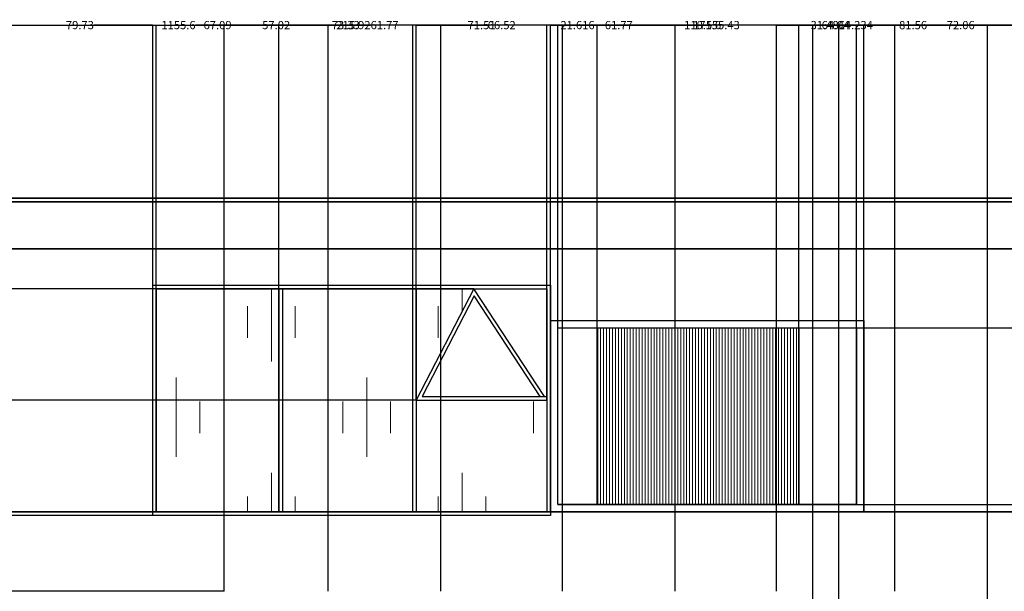
# Model space of a CAD drawing. Units: inches. Extents: x -1308 to 780, y 304 to 1023.
# Tile 6 of 7: x -138 to 402, y 709 to 1023. Entities that reach past the tile are written whole.
import ezdxf

# ---------------------------------------------------------------- set-up
doc = ezdxf.new("R2010")
doc.units = ezdxf.units.IN
doc.header["$MEASUREMENT"] = 0
for name, color, linetype, lineweight in [('A-ANNO-DIMS', 2, 'Continuous', 18), ('A-ELEV', 7, 'Continuous', 35), ('A-ELEV-PATT', 8, 'Continuous', 13), ('A-GLAZ', 4, 'Continuous', 25)]:
    doc.layers.add(name, color=color, linetype=linetype, lineweight=lineweight)
doc.styles.get("Standard").update_dxf_attribs({"font": 'arial.ttf'})
doc.dimstyles.get("Standard").update_dxf_attribs({"dimtxt": 4.5, "dimasz": 0.18, "dimexe": 0.18, "dimexo": 0.0625, "dimgap": 0.09, "dimtad": 0, "dimtih": 1, "dimtoh": 1, "dimdec": 4, "dimzin": 0, "dimdsep": 46, "dimlunit": 4, "dimtxsty": 'Standard', "dimcen": 0.09, "dimadec": 0, "dimazin": 0, "dimtfac": 1, "dimtdec": 4, "dimtofl": 0, "dimtmove": 0, "dimatfit": 3, "dimfxl": 1, "dimtolj": 1, "dimtzin": 0, "dimarcsym": 0})

# ---------------------------------------------------------------- blocks, each defined once
blk = doc.blocks.new('*D18')
at = {"layer": 'A-ANNO-DIMS', "color": 0, "lineweight": -2, "transparency": 16777216}
for p, q in [((-628.68, 924.9), (-628.68, 1019.77)), ((-628.5, 1019.59), (-60.08, 1019.59)), ((526.78, 1019.59), (-41.64, 1019.59)), ((526.96, 924.9), (526.96, 1019.77))]:
    blk.add_line(p, q, dxfattribs=at)
at = {"layer": 'A-ANNO-DIMS', "color": 0, "transparency": 16777216}
for points in [[(-628.5, 1019.62), (-628.5, 1019.56), (-628.68, 1019.59)], [(526.78, 1019.62), (526.78, 1019.56), (526.96, 1019.59)]]:
    blk.add_solid(points, dxfattribs=at)
at = {"layer": 'Defpoints', "color": 0, "transparency": 16777216}
for p in [(526.96, 1019.59), (-628.68, 924.84), (526.96, 924.84)]:
    blk.add_point(p, dxfattribs=at)
at = {"layer": 'A-ANNO-DIMS', "color": 0, "transparency": 16777216, "insert": (-50.86, 1019.59), "char_height": 4.5, "attachment_point": 5}
blk.add_mtext('\\A1;1155.6', dxfattribs=at)
blk = doc.blocks.new('*D27')
at = {"layer": 'A-ANNO-DIMS', "color": 0, "lineweight": -2, "transparency": 16777216}
for p, q in [((-144.73, 753.1), (-144.73, 1019.77)), ((-144.55, 1019.59), (-112.53, 1019.59)), ((-65.19, 1019.59), (-97.21, 1019.59)), ((-65.01, 751.1), (-65.01, 1019.77))]:
    blk.add_line(p, q, dxfattribs=at)
at = {"layer": 'A-ANNO-DIMS', "color": 0, "transparency": 16777216}
for points in [[(-144.55, 1019.62), (-144.55, 1019.56), (-144.73, 1019.59)], [(-65.19, 1019.62), (-65.19, 1019.56), (-65.01, 1019.59)]]:
    blk.add_solid(points, dxfattribs=at)
at = {"layer": 'Defpoints', "color": 0, "transparency": 16777216}
for p in [(-65.01, 1019.59), (-144.73, 753.04), (-65.01, 751.04)]:
    blk.add_point(p, dxfattribs=at)
at = {"layer": 'A-ANNO-DIMS', "color": 0, "transparency": 16777216, "insert": (-104.87, 1019.59), "char_height": 4.5, "attachment_point": 5}
blk.add_mtext('\\A1;79.73', dxfattribs=at)
blk = doc.blocks.new('*D28')
at = {"layer": 'A-ANNO-DIMS', "color": 0, "lineweight": -2, "transparency": 16777216}
for p, q in [((-63.01, 875.23), (-63.01, 1019.77)), ((-62.83, 1019.59), (35.51, 1019.59)), ((152.73, 1019.59), (54.4, 1019.59)), ((152.91, 877.23), (152.91, 1019.77))]:
    blk.add_line(p, q, dxfattribs=at)
at = {"layer": 'A-ANNO-DIMS', "color": 0, "transparency": 16777216}
for points in [[(-62.83, 1019.62), (-62.83, 1019.56), (-63.01, 1019.59)], [(152.73, 1019.62), (152.73, 1019.56), (152.91, 1019.59)]]:
    blk.add_solid(points, dxfattribs=at)
at = {"layer": 'Defpoints', "color": 0, "transparency": 16777216}
for p in [(152.91, 1019.59), (-63.01, 875.17), (152.91, 877.17)]:
    blk.add_point(p, dxfattribs=at)
at = {"layer": 'A-ANNO-DIMS', "color": 0, "transparency": 16777216, "insert": (44.95, 1019.59), "char_height": 4.5, "attachment_point": 5}
blk.add_mtext('\\A1;215.92', dxfattribs=at)
blk = doc.blocks.new('*D29')
at = {"layer": 'A-ANNO-DIMS', "color": 0, "lineweight": -2, "transparency": 16777216}
for p, q in [((-63.01, 753.1), (-63.01, 1019.77)), ((-62.83, 1019.59), (-37.16, 1019.59)), ((3.9, 1019.59), (-21.76, 1019.59)), ((4.08, 753.1), (4.08, 1019.77))]:
    blk.add_line(p, q, dxfattribs=at)
at = {"layer": 'A-ANNO-DIMS', "color": 0, "transparency": 16777216}
for points in [[(-62.83, 1019.62), (-62.83, 1019.56), (-63.01, 1019.59)], [(3.9, 1019.62), (3.9, 1019.56), (4.08, 1019.59)]]:
    blk.add_solid(points, dxfattribs=at)
at = {"layer": 'Defpoints', "color": 0, "transparency": 16777216}
for p in [(4.08, 1019.59), (-63.01, 753.04), (4.08, 753.04)]:
    blk.add_point(p, dxfattribs=at)
at = {"layer": 'A-ANNO-DIMS', "color": 0, "transparency": 16777216, "insert": (-29.46, 1019.59), "char_height": 4.5, "attachment_point": 5}
blk.add_mtext('\\A1;67.09', dxfattribs=at)
blk = doc.blocks.new('*D30')
at = {"layer": 'A-ANNO-DIMS', "color": 0, "lineweight": -2, "transparency": 16777216}
for p, q in [((4.08, 753.1), (4.08, 1019.77)), ((4.26, 1019.59), (33.08, 1019.59)), ((77.23, 1019.59), (48.41, 1019.59)), ((77.41, 753.1), (77.41, 1019.77))]:
    blk.add_line(p, q, dxfattribs=at)
at = {"layer": 'A-ANNO-DIMS', "color": 0, "transparency": 16777216}
for points in [[(4.26, 1019.62), (4.26, 1019.56), (4.08, 1019.59)], [(77.23, 1019.62), (77.23, 1019.56), (77.41, 1019.59)]]:
    blk.add_solid(points, dxfattribs=at)
at = {"layer": 'Defpoints', "color": 0, "transparency": 16777216}
for p in [(77.41, 1019.59), (4.08, 753.04), (77.41, 753.04)]:
    blk.add_point(p, dxfattribs=at)
at = {"layer": 'A-ANNO-DIMS', "color": 0, "transparency": 16777216, "insert": (40.74, 1019.59), "char_height": 4.5, "attachment_point": 5}
blk.add_mtext('\\A1;73.33', dxfattribs=at)
blk = doc.blocks.new('*D31')
at = {"layer": 'A-ANNO-DIMS', "color": 0, "lineweight": -2, "transparency": 16777216}
for p, q in [((79.41, 814.17), (79.41, 1019.77)), ((79.59, 1019.59), (107.93, 1019.59)), ((150.73, 1019.59), (122.39, 1019.59)), ((150.91, 814.17), (150.91, 1019.77))]:
    blk.add_line(p, q, dxfattribs=at)
at = {"layer": 'A-ANNO-DIMS', "color": 0, "transparency": 16777216}
for points in [[(79.59, 1019.62), (79.59, 1019.56), (79.41, 1019.59)], [(150.73, 1019.62), (150.73, 1019.56), (150.91, 1019.59)]]:
    blk.add_solid(points, dxfattribs=at)
at = {"layer": 'Defpoints', "color": 0, "transparency": 16777216}
for p in [(150.91, 1019.59), (79.41, 814.1), (150.91, 814.1)]:
    blk.add_point(p, dxfattribs=at)
at = {"layer": 'A-ANNO-DIMS', "color": 0, "transparency": 16777216, "insert": (115.16, 1019.59), "char_height": 4.5, "attachment_point": 5}
blk.add_mtext('\\A1;71.51', dxfattribs=at)
blk = doc.blocks.new('*D32')
at = {"layer": 'A-ANNO-DIMS', "color": 0, "lineweight": -2, "transparency": 16777216}
for p, q in [((152.91, 857.81), (152.91, 1019.77)), ((153.09, 1019.59), (231.24, 1019.59)), ((324.33, 1019.59), (246.18, 1019.59)), ((324.51, 857.81), (324.51, 1019.77))]:
    blk.add_line(p, q, dxfattribs=at)
at = {"layer": 'A-ANNO-DIMS', "color": 0, "transparency": 16777216}
for points in [[(153.09, 1019.62), (153.09, 1019.56), (152.91, 1019.59)], [(324.33, 1019.62), (324.33, 1019.56), (324.51, 1019.59)]]:
    blk.add_solid(points, dxfattribs=at)
at = {"layer": 'Defpoints', "color": 0, "transparency": 16777216}
for p in [(324.51, 1019.59), (152.91, 857.74), (324.51, 857.74)]:
    blk.add_point(p, dxfattribs=at)
at = {"layer": 'A-ANNO-DIMS', "color": 0, "transparency": 16777216, "insert": (238.71, 1019.59), "char_height": 4.5, "attachment_point": 5}
blk.add_mtext('\\A1;171.6', dxfattribs=at)
blk = doc.blocks.new('*D33')
at = {"layer": 'A-ANNO-DIMS', "color": 0, "lineweight": -2, "transparency": 16777216}
for p, q in [((156.91, 757.1), (156.91, 1019.77)), ((157.09, 1019.59), (158.26, 1019.59)), ((178.35, 1019.59), (177.19, 1019.59)), ((178.53, 757.1), (178.53, 1019.77))]:
    blk.add_line(p, q, dxfattribs=at)
at = {"layer": 'A-ANNO-DIMS', "color": 0, "transparency": 16777216}
for points in [[(157.09, 1019.62), (157.09, 1019.56), (156.91, 1019.59)], [(178.35, 1019.62), (178.35, 1019.56), (178.53, 1019.59)]]:
    blk.add_solid(points, dxfattribs=at)
at = {"layer": 'Defpoints', "color": 0, "transparency": 16777216}
for p in [(178.53, 1019.59), (156.91, 757.04), (178.53, 757.04)]:
    blk.add_point(p, dxfattribs=at)
at = {"layer": 'A-ANNO-DIMS', "color": 0, "transparency": 16777216, "insert": (167.72, 1019.59), "char_height": 4.5, "attachment_point": 5}
blk.add_mtext('\\A1;21.616', dxfattribs=at)
blk = doc.blocks.new('*D34')
at = {"layer": 'A-ANNO-DIMS', "color": 0, "lineweight": -2, "transparency": 16777216}
for p, q in [((178.53, 757.1), (178.53, 1019.77)), ((178.71, 1019.59), (226.29, 1019.59)), ((288.84, 1019.59), (241.26, 1019.59)), ((289.02, 757.1), (289.02, 1019.77))]:
    blk.add_line(p, q, dxfattribs=at)
at = {"layer": 'A-ANNO-DIMS', "color": 0, "transparency": 16777216}
for points in [[(178.71, 1019.62), (178.71, 1019.56), (178.53, 1019.59)], [(288.84, 1019.62), (288.84, 1019.56), (289.02, 1019.59)]]:
    blk.add_solid(points, dxfattribs=at)
at = {"layer": 'Defpoints', "color": 0, "transparency": 16777216}
for p in [(289.02, 1019.59), (178.53, 757.04), (289.02, 757.04)]:
    blk.add_point(p, dxfattribs=at)
at = {"layer": 'A-ANNO-DIMS', "color": 0, "transparency": 16777216, "insert": (233.78, 1019.59), "char_height": 4.5, "attachment_point": 5}
blk.add_mtext('\\A1;110.5', dxfattribs=at)
blk = doc.blocks.new('*D35')
at = {"layer": 'A-ANNO-DIMS', "color": 0, "lineweight": -2, "transparency": 16777216}
for p, q in [((289.02, 757.1), (289.02, 1019.77)), ((289.2, 1019.59), (295.34, 1019.59)), ((320.33, 1019.59), (314.19, 1019.59)), ((320.51, 757.1), (320.51, 1019.77))]:
    blk.add_line(p, q, dxfattribs=at)
at = {"layer": 'A-ANNO-DIMS', "color": 0, "transparency": 16777216}
for points in [[(289.2, 1019.62), (289.2, 1019.56), (289.02, 1019.59)], [(320.33, 1019.62), (320.33, 1019.56), (320.51, 1019.59)]]:
    blk.add_solid(points, dxfattribs=at)
at = {"layer": 'Defpoints', "color": 0, "transparency": 16777216}
for p in [(320.51, 1019.59), (289.02, 757.04), (320.51, 757.04)]:
    blk.add_point(p, dxfattribs=at)
at = {"layer": 'A-ANNO-DIMS', "color": 0, "transparency": 16777216, "insert": (304.76, 1019.59), "char_height": 4.5, "attachment_point": 5}
blk.add_mtext('\\A1;31.486', dxfattribs=at)
blk = doc.blocks.new('*D36')
at = {"layer": 'A-ANNO-DIMS', "color": 0, "lineweight": -2, "transparency": 16777216}
for p, q in [((324.51, 753.1), (324.51, 1019.77)), ((324.69, 1019.59), (416.25, 1019.59)), ((526.78, 1019.59), (435.22, 1019.59)), ((526.96, 753.1), (526.96, 1019.77))]:
    blk.add_line(p, q, dxfattribs=at)
at = {"layer": 'A-ANNO-DIMS', "color": 0, "transparency": 16777216}
for points in [[(324.69, 1019.62), (324.69, 1019.56), (324.51, 1019.59)], [(526.78, 1019.62), (526.78, 1019.56), (526.96, 1019.59)]]:
    blk.add_solid(points, dxfattribs=at)
at = {"layer": 'Defpoints', "color": 0, "transparency": 16777216}
for p in [(526.96, 1019.59), (324.51, 753.04), (526.96, 753.04)]:
    blk.add_point(p, dxfattribs=at)
at = {"layer": 'A-ANNO-DIMS', "color": 0, "transparency": 16777216, "insert": (425.73, 1019.59), "char_height": 4.5, "attachment_point": 5}
blk.add_mtext('\\A1;202.45', dxfattribs=at)
blk = doc.blocks.new('*D37')
at = {"layer": 'A-ANNO-DIMS', "color": 0, "lineweight": -2, "transparency": 16777216}
for p, q in [((-25.86, 709.52), (-25.86, 1019.77)), ((-25.68, 1019.59), (-5.01, 1019.59)), ((30.98, 1019.59), (10.31, 1019.59)), ((31.16, 709.52), (31.16, 1019.77))]:
    blk.add_line(p, q, dxfattribs=at)
at = {"layer": 'A-ANNO-DIMS', "color": 0, "transparency": 16777216}
for points in [[(-25.68, 1019.62), (-25.68, 1019.56), (-25.86, 1019.59)], [(30.98, 1019.62), (30.98, 1019.56), (31.16, 1019.59)]]:
    blk.add_solid(points, dxfattribs=at)
at = {"layer": 'Defpoints', "color": 0, "transparency": 16777216}
for p in [(31.16, 1019.59), (-25.86, 709.46), (31.16, 709.46)]:
    blk.add_point(p, dxfattribs=at)
at = {"layer": 'A-ANNO-DIMS', "color": 0, "transparency": 16777216, "insert": (2.65, 1019.59), "char_height": 4.5, "attachment_point": 5}
blk.add_mtext('\\A1;57.02', dxfattribs=at)
blk = doc.blocks.new('*D38')
at = {"layer": 'A-ANNO-DIMS', "color": 0, "lineweight": -2, "transparency": 16777216}
for p, q in [((31.16, 709.52), (31.16, 1019.77)), ((31.34, 1019.59), (54.35, 1019.59)), ((92.75, 1019.59), (69.74, 1019.59)), ((92.93, 709.52), (92.93, 1019.77))]:
    blk.add_line(p, q, dxfattribs=at)
at = {"layer": 'A-ANNO-DIMS', "color": 0, "transparency": 16777216}
for points in [[(31.34, 1019.62), (31.34, 1019.56), (31.16, 1019.59)], [(92.75, 1019.62), (92.75, 1019.56), (92.93, 1019.59)]]:
    blk.add_solid(points, dxfattribs=at)
at = {"layer": 'Defpoints', "color": 0, "transparency": 16777216}
for p in [(92.93, 1019.59), (31.16, 709.46), (92.93, 709.46)]:
    blk.add_point(p, dxfattribs=at)
at = {"layer": 'A-ANNO-DIMS', "color": 0, "transparency": 16777216, "insert": (62.04, 1019.59), "char_height": 4.5, "attachment_point": 5}
blk.add_mtext('\\A1;61.77', dxfattribs=at)
blk = doc.blocks.new('*D39')
at = {"layer": 'A-ANNO-DIMS', "color": 0, "lineweight": -2, "transparency": 16777216}
for p, q in [((92.93, 709.52), (92.93, 1019.77)), ((93.11, 1019.59), (118.52, 1019.59)), ((159.27, 1019.59), (133.86, 1019.59)), ((159.45, 709.52), (159.45, 1019.77))]:
    blk.add_line(p, q, dxfattribs=at)
at = {"layer": 'A-ANNO-DIMS', "color": 0, "transparency": 16777216}
for points in [[(93.11, 1019.62), (93.11, 1019.56), (92.93, 1019.59)], [(159.27, 1019.62), (159.27, 1019.56), (159.45, 1019.59)]]:
    blk.add_solid(points, dxfattribs=at)
at = {"layer": 'Defpoints', "color": 0, "transparency": 16777216}
for p in [(159.45, 1019.59), (92.93, 709.46), (159.45, 709.46)]:
    blk.add_point(p, dxfattribs=at)
at = {"layer": 'A-ANNO-DIMS', "color": 0, "transparency": 16777216, "insert": (126.19, 1019.59), "char_height": 4.5, "attachment_point": 5}
blk.add_mtext('\\A1;66.52', dxfattribs=at)
blk = doc.blocks.new('*D40')
at = {"layer": 'A-ANNO-DIMS', "color": 0, "lineweight": -2, "transparency": 16777216}
for p, q in [((159.45, 709.52), (159.45, 1019.77)), ((159.63, 1019.59), (182.64, 1019.59)), ((221.04, 1019.59), (198.03, 1019.59)), ((221.22, 709.52), (221.22, 1019.77))]:
    blk.add_line(p, q, dxfattribs=at)
at = {"layer": 'A-ANNO-DIMS', "color": 0, "transparency": 16777216}
for points in [[(159.63, 1019.62), (159.63, 1019.56), (159.45, 1019.59)], [(221.04, 1019.62), (221.04, 1019.56), (221.22, 1019.59)]]:
    blk.add_solid(points, dxfattribs=at)
at = {"layer": 'Defpoints', "color": 0, "transparency": 16777216}
for p in [(221.22, 1019.59), (159.45, 709.46), (221.22, 709.46)]:
    blk.add_point(p, dxfattribs=at)
at = {"layer": 'A-ANNO-DIMS', "color": 0, "transparency": 16777216, "insert": (190.33, 1019.59), "char_height": 4.5, "attachment_point": 5}
blk.add_mtext('\\A1;61.77', dxfattribs=at)
blk = doc.blocks.new('*D41')
at = {"layer": 'A-ANNO-DIMS', "color": 0, "lineweight": -2, "transparency": 16777216}
for p, q in [((221.22, 709.52), (221.22, 1019.77)), ((221.4, 1019.59), (241.25, 1019.59)), ((276.47, 1019.59), (256.62, 1019.59)), ((276.65, 709.52), (276.65, 1019.77))]:
    blk.add_line(p, q, dxfattribs=at)
at = {"layer": 'A-ANNO-DIMS', "color": 0, "transparency": 16777216}
for points in [[(221.4, 1019.62), (221.4, 1019.56), (221.22, 1019.59)], [(276.47, 1019.62), (276.47, 1019.56), (276.65, 1019.59)]]:
    blk.add_solid(points, dxfattribs=at)
at = {"layer": 'Defpoints', "color": 0, "transparency": 16777216}
for p in [(276.65, 1019.59), (221.22, 709.46), (276.65, 709.46)]:
    blk.add_point(p, dxfattribs=at)
at = {"layer": 'A-ANNO-DIMS', "color": 0, "transparency": 16777216, "insert": (248.94, 1019.59), "char_height": 4.5, "attachment_point": 5}
blk.add_mtext('\\A1;55.43', dxfattribs=at)
blk = doc.blocks.new('*D42')
at = {"layer": 'A-ANNO-DIMS', "color": 0, "lineweight": -2, "transparency": 16777216}
for p, q in [((276.65, 709.52), (276.65, 1019.77)), ((276.83, 1019.59), (301.44, 1019.59)), ((341.41, 1019.59), (316.81, 1019.59)), ((341.59, 709.52), (341.59, 1019.77))]:
    blk.add_line(p, q, dxfattribs=at)
at = {"layer": 'A-ANNO-DIMS', "color": 0, "transparency": 16777216}
for points in [[(276.83, 1019.62), (276.83, 1019.56), (276.65, 1019.59)], [(341.41, 1019.62), (341.41, 1019.56), (341.59, 1019.59)]]:
    blk.add_solid(points, dxfattribs=at)
at = {"layer": 'Defpoints', "color": 0, "transparency": 16777216}
for p in [(341.59, 1019.59), (276.65, 709.46), (341.59, 709.46)]:
    blk.add_point(p, dxfattribs=at)
at = {"layer": 'A-ANNO-DIMS', "color": 0, "transparency": 16777216, "insert": (309.12, 1019.59), "char_height": 4.5, "attachment_point": 5}
blk.add_mtext('\\A1;64.94', dxfattribs=at)
blk = doc.blocks.new('*D43')
at = {"layer": 'A-ANNO-DIMS', "color": 0, "lineweight": -2, "transparency": 16777216}
for p, q in [((341.59, 709.52), (341.59, 1019.77)), ((341.77, 1019.59), (369.96, 1019.59)), ((413.47, 1019.59), (385.28, 1019.59)), ((413.65, 709.52), (413.65, 1019.77))]:
    blk.add_line(p, q, dxfattribs=at)
at = {"layer": 'A-ANNO-DIMS', "color": 0, "transparency": 16777216}
for points in [[(341.77, 1019.62), (341.77, 1019.56), (341.59, 1019.59)], [(413.47, 1019.62), (413.47, 1019.56), (413.65, 1019.59)]]:
    blk.add_solid(points, dxfattribs=at)
at = {"layer": 'Defpoints', "color": 0, "transparency": 16777216}
for p in [(413.65, 1019.59), (341.59, 709.46), (413.65, 709.46)]:
    blk.add_point(p, dxfattribs=at)
at = {"layer": 'A-ANNO-DIMS', "color": 0, "transparency": 16777216, "insert": (377.62, 1019.59), "char_height": 4.5, "attachment_point": 5}
blk.add_mtext('\\A1;72.06', dxfattribs=at)
blk = doc.blocks.new('*D55')
at = {"layer": 'A-ANNO-DIMS', "color": 0, "lineweight": -2, "transparency": 16777216}
for p, q in [((310.77, 463.5), (310.77, 1019.77)), ((310.95, 1019.59), (343.86, 1019.59)), ((392.14, 1019.59), (359.23, 1019.59)), ((392.32, 494.13), (392.32, 1019.77))]:
    blk.add_line(p, q, dxfattribs=at)
at = {"layer": 'A-ANNO-DIMS', "color": 0, "transparency": 16777216}
for points in [[(310.95, 1019.62), (310.95, 1019.56), (310.77, 1019.59)], [(392.14, 1019.62), (392.14, 1019.56), (392.32, 1019.59)]]:
    blk.add_solid(points, dxfattribs=at)
at = {"layer": 'Defpoints', "color": 0, "transparency": 16777216}
for p in [(392.32, 1019.59), (392.32, 494.07), (310.77, 463.43)]:
    blk.add_point(p, dxfattribs=at)
at = {"layer": 'A-ANNO-DIMS', "color": 0, "transparency": 16777216, "insert": (351.54, 1019.59), "char_height": 4.5, "attachment_point": 5}
blk.add_mtext('\\A1;81.56', dxfattribs=at)
blk = doc.blocks.new('*D56')
at = {"layer": 'A-ANNO-DIMS', "color": 0, "lineweight": -2, "transparency": 16777216}
for p, q in [((296.53, 402.08), (296.53, 1019.77)), ((296.71, 1019.59), (310.59, 1019.59)), ((310.77, 463.5), (310.77, 1019.77)), ((310.77, 1019.59), (310.95, 1019.59))]:
    blk.add_line(p, q, dxfattribs=at)
at = {"layer": 'A-ANNO-DIMS', "color": 0, "transparency": 16777216}
for points in [[(296.71, 1019.62), (296.71, 1019.56), (296.53, 1019.59)], [(310.59, 1019.62), (310.59, 1019.56), (310.77, 1019.59)]]:
    blk.add_solid(points, dxfattribs=at)
at = {"layer": 'Defpoints', "color": 0, "transparency": 16777216}
for p in [(310.77, 1019.59), (310.77, 463.43), (296.53, 402.02)]:
    blk.add_point(p, dxfattribs=at)
at = {"layer": 'A-ANNO-DIMS', "color": 0, "transparency": 16777216, "insert": (320.15, 1019.59), "char_height": 4.5, "attachment_point": 5}
blk.add_mtext('\\A1;14.234', dxfattribs=at)
blk = doc.blocks.new('*D65')
at = {"layer": 'A-ANNO-DIMS', "color": 0, "lineweight": -2, "transparency": 16777216}
for p, q in [((-843.54, 753.04), (771.09, 753.04)), ((770.91, 752.86), (770.91, 730.95)), ((770.91, 704.27), (770.91, 726.17)), ((-843.54, 704.09), (771.09, 704.09))]:
    blk.add_line(p, q, dxfattribs=at)
at = {"layer": 'A-ANNO-DIMS', "color": 0, "transparency": 16777216}
for points in [[(770.88, 752.86), (770.94, 752.86), (770.91, 753.04)], [(770.88, 704.27), (770.94, 704.27), (770.91, 704.09)]]:
    blk.add_solid(points, dxfattribs=at)
at = {"layer": 'Defpoints', "color": 0, "transparency": 16777216}
for p in [(-843.6, 753.04), (770.91, 753.04), (-843.6, 704.09)]:
    blk.add_point(p, dxfattribs=at)
at = {"layer": 'A-ANNO-DIMS', "color": 0, "transparency": 16777216, "insert": (770.91, 728.56), "char_height": 4.5, "attachment_point": 5}
blk.add_mtext('\\A1;48.95', dxfattribs=at)
blk = doc.blocks.new('*D82')
at = {"layer": 'A-ANNO-DIMS', "color": 0, "lineweight": -2, "transparency": 16777216}
for p, q in [((-25.92, 709.46), (-1298.45, 709.46)), ((-1298.27, 709.28), (-1298.27, 664.37)), ((-1298.27, 614.69), (-1298.27, 659.6)), ((-25.92, 614.51), (-1298.45, 614.51))]:
    blk.add_line(p, q, dxfattribs=at)
at = {"layer": 'A-ANNO-DIMS', "color": 0, "transparency": 16777216}
for points in [[(-1298.3, 709.28), (-1298.24, 709.28), (-1298.27, 709.46)], [(-1298.3, 614.69), (-1298.24, 614.69), (-1298.27, 614.51)]]:
    blk.add_solid(points, dxfattribs=at)
at = {"layer": 'Defpoints', "color": 0, "transparency": 16777216}
for p in [(-1298.27, 709.46), (-25.86, 709.46), (-25.86, 614.51)]:
    blk.add_point(p, dxfattribs=at)
at = {"layer": 'A-ANNO-DIMS', "color": 0, "transparency": 16777216, "insert": (-1298.27, 661.98), "char_height": 4.5, "attachment_point": 5}
blk.add_mtext('\\A1;94.95', dxfattribs=at)
blk = doc.blocks.new('*D83')
at = {"layer": 'A-ANNO-DIMS', "color": 0, "lineweight": -2, "transparency": 16777216}
for p, q in [((4.02, 753.04), (-1298.45, 753.04)), ((-1298.27, 752.86), (-1298.27, 733.64)), ((-1298.27, 709.64), (-1298.27, 728.86)), ((-25.92, 709.46), (-1298.45, 709.46))]:
    blk.add_line(p, q, dxfattribs=at)
at = {"layer": 'A-ANNO-DIMS', "color": 0, "transparency": 16777216}
for points in [[(-1298.3, 752.86), (-1298.24, 752.86), (-1298.27, 753.04)], [(-1298.3, 709.64), (-1298.24, 709.64), (-1298.27, 709.46)]]:
    blk.add_solid(points, dxfattribs=at)
at = {"layer": 'Defpoints', "color": 0, "transparency": 16777216}
for p in [(-1298.27, 753.04), (4.08, 753.04), (-25.86, 709.46)]:
    blk.add_point(p, dxfattribs=at)
at = {"layer": 'A-ANNO-DIMS', "color": 0, "transparency": 16777216, "insert": (-1298.27, 731.25), "char_height": 4.5, "attachment_point": 5}
blk.add_mtext('\\A1;43.58', dxfattribs=at)
blk = doc.blocks.new('*D85')
at = {"layer": 'A-ANNO-DIMS', "color": 0, "lineweight": -2, "transparency": 16777216}
for p, q in [((-63.07, 875.17), (-1298.45, 875.17)), ((-1298.27, 874.99), (-1298.27, 815.49)), ((-1298.27, 751.22), (-1298.27, 810.72)), ((-65.07, 751.04), (-1298.45, 751.04))]:
    blk.add_line(p, q, dxfattribs=at)
at = {"layer": 'A-ANNO-DIMS', "color": 0, "transparency": 16777216}
for points in [[(-1298.3, 874.99), (-1298.24, 874.99), (-1298.27, 875.17)], [(-1298.3, 751.22), (-1298.24, 751.22), (-1298.27, 751.04)]]:
    blk.add_solid(points, dxfattribs=at)
at = {"layer": 'Defpoints', "color": 0, "transparency": 16777216}
for p in [(-1298.27, 875.17), (-63.01, 875.17), (-65.01, 751.04)]:
    blk.add_point(p, dxfattribs=at)
at = {"layer": 'A-ANNO-DIMS', "color": 0, "transparency": 16777216, "insert": (-1298.27, 813.1), "char_height": 4.5, "attachment_point": 5}
blk.add_mtext('\\A1;124.13', dxfattribs=at)
blk = doc.blocks.new('*D86')
at = {"layer": 'A-ANNO-DIMS', "color": 0, "lineweight": -2, "transparency": 16777216}
for p, q in [((79.34, 814.1), (-1298.45, 814.1)), ((-1298.27, 813.92), (-1298.27, 785.96)), ((-1298.27, 753.22), (-1298.27, 781.18)), ((79.34, 753.04), (-1298.45, 753.04))]:
    blk.add_line(p, q, dxfattribs=at)
at = {"layer": 'A-ANNO-DIMS', "color": 0, "transparency": 16777216}
for points in [[(-1298.3, 813.92), (-1298.24, 813.92), (-1298.27, 814.1)], [(-1298.3, 753.22), (-1298.24, 753.22), (-1298.27, 753.04)]]:
    blk.add_solid(points, dxfattribs=at)
at = {"layer": 'Defpoints', "color": 0, "transparency": 16777216}
for p in [(-1298.27, 814.1), (79.41, 814.1), (79.41, 753.04)]:
    blk.add_point(p, dxfattribs=at)
at = {"layer": 'A-ANNO-DIMS', "color": 0, "transparency": 16777216, "insert": (-1298.27, 783.57), "char_height": 4.5, "attachment_point": 5}
blk.add_mtext('\\A1;61.07', dxfattribs=at)
blk = doc.blocks.new('*D87')
at = {"layer": 'A-ANNO-DIMS', "color": 0, "lineweight": -2, "transparency": 16777216}
for p, q in [((110.86, 875.17), (-1298.45, 875.17)), ((-1298.27, 874.99), (-1298.27, 847.03)), ((-1298.27, 814.28), (-1298.27, 842.25)), ((79.34, 814.1), (-1298.45, 814.1))]:
    blk.add_line(p, q, dxfattribs=at)
at = {"layer": 'A-ANNO-DIMS', "color": 0, "transparency": 16777216}
for points in [[(-1298.3, 874.99), (-1298.24, 874.99), (-1298.27, 875.17)], [(-1298.3, 814.28), (-1298.24, 814.28), (-1298.27, 814.1)]]:
    blk.add_solid(points, dxfattribs=at)
at = {"layer": 'Defpoints', "color": 0, "transparency": 16777216}
for p in [(-1298.27, 875.17), (110.92, 875.17), (79.41, 814.1)]:
    blk.add_point(p, dxfattribs=at)
at = {"layer": 'A-ANNO-DIMS', "color": 0, "transparency": 16777216, "insert": (-1298.27, 844.64), "char_height": 4.5, "attachment_point": 5}
blk.add_mtext('\\A1;61.07', dxfattribs=at)
blk = doc.blocks.new('*D88')
at = {"layer": 'A-ANNO-DIMS', "color": 0, "lineweight": -2, "transparency": 16777216}
for p, q in [((156.98, 853.74), (771.09, 853.74)), ((770.91, 853.56), (770.91, 807.78)), ((770.91, 757.22), (770.91, 803)), ((156.98, 757.04), (771.09, 757.04))]:
    blk.add_line(p, q, dxfattribs=at)
at = {"layer": 'A-ANNO-DIMS', "color": 0, "transparency": 16777216}
for points in [[(770.88, 853.56), (770.94, 853.56), (770.91, 853.74)], [(770.88, 757.22), (770.94, 757.22), (770.91, 757.04)]]:
    blk.add_solid(points, dxfattribs=at)
at = {"layer": 'Defpoints', "color": 0, "transparency": 16777216}
for p in [(156.91, 853.74), (770.91, 853.74), (156.91, 757.04)]:
    blk.add_point(p, dxfattribs=at)
at = {"layer": 'A-ANNO-DIMS', "color": 0, "transparency": 16777216, "insert": (770.91, 805.39), "char_height": 4.5, "attachment_point": 5}
blk.add_mtext('\\A1;96.7', dxfattribs=at)

msp = doc.modelspace()

# ---------------------------------------------------------------- hatches: boundary and pattern name
at = {"layer": 'A-ELEV-PATT'}
h = msp.add_hatch(dxfattribs=at)
h.set_pattern_fill('GOST_GLASS', color=256, scale=8.7, angle=45)
h.set_pattern_definition([(90, (0, 0), (52.2, 52.2), [43.5, -60.9]), (90, (13.05, 13.05), (52.2, 52.2), [17.4, -87]), (90, (-13.05, 13.05), (52.2, 52.2), [17.4, -87])])
h.paths.add_polyline_path([(-570.795, 854.0948), (-613.9558, 854.0948), (-613.9558, 755.0385), (-570.795, 755.0385)])
h.paths.add_polyline_path([(-499.4748, 854.0948), (-568.795, 854.0948), (-568.795, 755.0385), (-499.4748, 755.0385)])
h.paths.add_polyline_path([(-379.8352, 854.0948), (-497.4748, 854.0948), (-497.4748, 755.0385), (-379.8352, 755.0385)])
h.paths.add_polyline_path([(-292.4461, 854.0948), (-377.8352, 854.0948), (-377.8352, 755.0385), (-292.4461, 755.0385)])
h.paths.add_polyline_path([(4.0783, 875.1709), (-63.0069, 875.1709), (-63.0069, 753.0385), (4.0783, 753.0385)])
h.paths.add_polyline_path([(77.4055, 875.1709), (6.0783, 875.1709), (6.0783, 753.0385), (77.4055, 753.0385)])
h.paths.add_polyline_path([(150.9148, 814.1047), (79.4055, 814.1047), (79.4055, 753.0385), (150.9148, 753.0385)])
h.paths.add_polyline_path([(110.9181, 875.1709), (79.4055, 875.1709), (79.4055, 814.1047)])
h.paths.add_polyline_path([(150.9148, 875.1709), (110.9181, 875.1709), (149.6048, 816.1047), (150.9148, 816.1047)])
h.paths.add_polyline_path([(-227.6882, 875.1709), (-271.346, 875.1709), (-271.346, 753.0385), (-227.6882, 753.0385)])
h.paths.add_polyline_path([(-188.3907, 875.1709), (-227.6882, 875.1709), (-227.6882, 753.0385), (-188.3907, 753.0385)])
h.paths.add_polyline_path([(-144.7329, 875.1709), (-188.3907, 875.1709), (-188.3907, 753.0385), (-144.7329, 753.0385)])
h.paths.add_polyline_path([(-144.7329, 739.0259), (-188.3907, 739.0259), (-188.3907, 624.4429), (-144.7329, 624.4429)])
h.paths.add_polyline_path([(-188.3907, 739.0259), (-227.6882, 739.0259), (-227.6882, 624.4429), (-188.3907, 624.4429)])
h.paths.add_polyline_path([(-227.6882, 739.0259), (-271.346, 739.0259), (-271.346, 624.4429), (-227.6882, 624.4429)])
h.paths.add_polyline_path([(-229.1416, 600.0434), (-271.346, 600.0434), (-271.346, 411.1006), (-229.1416, 411.1006)])
h.paths.add_polyline_path([(-186.9373, 600.0434), (-229.1416, 600.0434), (-229.1416, 411.1006), (-186.9373, 411.1006)])
h.paths.add_polyline_path([(-144.7329, 600.0434), (-186.9373, 600.0434), (-186.9373, 411.1006), (-144.7329, 411.1006)])
h = msp.add_hatch(dxfattribs=at)
h.set_pattern_fill('ANSI31', color=256, scale=13, angle=45)
h.paths.add_polyline_path([(289.0202, 853.744), (178.5305, 853.744), (178.5305, 757.0385), (289.0202, 757.0385)])

# ---------------------------------------------------------------- linework, layer by layer
at = {"layer": 'A-ELEV'}
for p, q in [((-628.6809, 924.8421), (381.6743, 924.8421)), ((-628.6809, 922.8421), (381.6743, 922.8421)), ((381.6743, 924.8421), (526.9606, 924.8421)), ((381.6743, 922.8421), (526.9606, 922.8421)), ((-130.9821, 897.0385), (-144.7329, 897.0385)), ((-130.9821, 897.0385), (226.3529, 897.0385)), ((226.3529, 897.0385), (526.9606, 897.0385)), ((526.9606, 753.0385), (-144.7329, 753.0385))]:
    msp.add_line(p, q, dxfattribs=at)
at = {"layer": 'A-GLAZ'}
for p, q in [((4.0783, 875.1709), (4.0783, 753.0385)), ((6.0783, 875.1709), (6.0783, 753.0385)), ((77.4055, 875.1709), (77.4055, 753.0385)), ((79.4055, 875.1709), (79.4055, 753.0385)), ((110.9181, 875.1709), (79.4055, 814.1047)), ((149.6048, 816.1047), (110.9181, 875.1709)), ((111.1233, 871.2074), (82.6882, 816.1047)), ((147.214, 816.1047), (111.1233, 871.2074)), ((178.5305, 853.744), (178.5305, 757.0385)), ((289.0202, 853.744), (289.0202, 757.0385)), ((82.6882, 816.1047), (150.9148, 816.1047)), ((79.4055, 814.1047), (150.9148, 814.1047))]:
    msp.add_line(p, q, dxfattribs=at)
for points in [[(-65.0069, 877.1709), (152.9148, 877.1709), (152.9148, 751.0385), (-65.0069, 751.0385)], [(-63.0069, 875.1709), (150.9148, 875.1709), (150.9148, 753.0385), (-63.0069, 753.0385)], [(152.9148, 857.744), (324.5059, 857.744), (324.5059, 753.0385), (152.9148, 753.0385)], [(156.9148, 853.744), (320.5059, 853.744), (320.5059, 757.0385), (156.9148, 757.0385)]]:
    msp.add_lwpolyline(points, close=True, dxfattribs=at)

# ---------------------------------------------------------------- dimensions: what is measured, and where the dimension line sits
at = {"layer": 'A-ANNO-DIMS'}
for base, p1, p2, override, picture, middle in [((526.9606, 1019.5921), (-628.6809, 924.8421), (526.9606, 924.8421), {"dimdec": 1, "dimlfac": 1, "dimrnd": 0, "dimzin": 0, "dimdsep": 46, "dimlunit": 2}, '*D18', (-50.8601, 1019.5921)), ((-65.0069, 1019.5921), (-144.7329, 753.0385), (-65.0069, 751.0385), {"dimdec": 2, "dimlfac": 1, "dimrnd": 0, "dimzin": 0, "dimdsep": 46, "dimlunit": 2}, '*D27', (-104.8699, 1019.5921)), ((152.9148, 1019.5921), (-63.0069, 875.1709), (152.9148, 877.1709), {"dimdec": 2, "dimlfac": 1, "dimrnd": 0, "dimzin": 0, "dimdsep": 46, "dimlunit": 2}, '*D28', (44.9539, 1019.5921)), ((4.0783, 1019.5921), (-63.0069, 753.0385), (4.0783, 753.0385), {"dimdec": 2, "dimlfac": 1, "dimrnd": 0, "dimzin": 0, "dimdsep": 46, "dimlunit": 2}, '*D29', (-29.4643, 1019.5921)), ((31.1601, 1019.5921), (-25.8575, 709.4602), (31.1601, 709.4602), {"dimdec": 2, "dimlfac": 1, "dimrnd": 0, "dimzin": 0, "dimdsep": 46, "dimlunit": 2}, '*D37', (2.6513, 1019.5921)), ((77.4055, 1019.5921), (4.0783, 753.0385), (77.4055, 753.0385), {"dimdec": 2, "dimlfac": 1, "dimrnd": 0, "dimzin": 0, "dimdsep": 46, "dimlunit": 2}, '*D30', (40.7419, 1019.5921)), ((92.9293, 1019.5921), (31.1601, 709.4602), (92.9293, 709.4602), {"dimdec": 2, "dimlfac": 1, "dimrnd": 0, "dimzin": 0, "dimdsep": 46, "dimlunit": 2}, '*D38', (62.0447, 1019.5921)), ((150.9148, 1019.5921), (79.4055, 814.1047), (150.9148, 814.1047), {"dimdec": 2, "dimlfac": 1, "dimrnd": 0, "dimzin": 0, "dimdsep": 46, "dimlunit": 2}, '*D31', (115.1602, 1019.5921)), ((159.4499, 1019.5921), (92.9293, 709.4602), (159.4499, 709.4602), {"dimdec": 2, "dimlfac": 1, "dimrnd": 0, "dimzin": 0, "dimdsep": 46, "dimlunit": 2}, '*D39', (126.1896, 1019.5921)), ((324.5059, 1019.5921), (152.9148, 857.744), (324.5059, 857.744), {"dimdec": 1, "dimlfac": 1, "dimrnd": 0, "dimzin": 0, "dimdsep": 46, "dimlunit": 2}, '*D32', (238.7103, 1019.5921)), ((178.5305, 1019.5921), (156.9148, 757.0385), (178.5305, 757.0385), {"dimdec": 3, "dimlfac": 1, "dimrnd": 0, "dimzin": 0, "dimdsep": 46, "dimlunit": 2}, '*D33', (167.7226, 1019.5921)), ((221.219, 1019.5921), (159.4499, 709.4602), (221.219, 709.4602), {"dimdec": 2, "dimlfac": 1, "dimrnd": 0, "dimzin": 0, "dimdsep": 46, "dimlunit": 2}, '*D40', (190.3345, 1019.5921)), ((289.0202, 1019.5921), (178.5305, 757.0385), (289.0202, 757.0385), {"dimdec": 1, "dimlfac": 1, "dimrnd": 0, "dimzin": 0, "dimdsep": 46, "dimlunit": 2}, '*D34', (233.7754, 1019.5921)), ((276.6529, 1019.5921), (221.219, 709.4602), (276.6529, 709.4602), {"dimdec": 2, "dimlfac": 1, "dimrnd": 0, "dimzin": 0, "dimdsep": 46, "dimlunit": 2}, '*D41', (248.9359, 1019.5921)), ((341.5897, 1019.5921), (276.6529, 709.4602), (341.5897, 709.4602), {"dimdec": 2, "dimlfac": 1, "dimrnd": 0, "dimzin": 0, "dimdsep": 46, "dimlunit": 2}, '*D42', (309.1213, 1019.5921)), ((320.5059, 1019.5921), (289.0202, 757.0385), (320.5059, 757.0385), {"dimdec": 3, "dimlfac": 1, "dimrnd": 0, "dimzin": 0, "dimdsep": 46, "dimlunit": 2}, '*D35', (304.763, 1019.5921)), ((310.7651, 1019.5921), (296.5309, 402.0158), (310.7651, 463.4331), {"dimdec": 3, "dimlfac": 1, "dimrnd": 0, "dimzin": 0, "dimdsep": 46, "dimlunit": 2}, '*D56', (320.1548, 1019.5921)), ((392.3226, 1019.5921), (310.7651, 463.4331), (392.3226, 494.0703), {"dimdec": 2, "dimlfac": 1, "dimrnd": 0, "dimzin": 0, "dimdsep": 46, "dimlunit": 2}, '*D55', (351.5439, 1019.5921)), ((526.9606, 1019.5921), (324.5059, 753.0385), (526.9606, 753.0385), {"dimdec": 2, "dimlfac": 1, "dimrnd": 0, "dimzin": 0, "dimdsep": 46, "dimlunit": 2}, '*D36', (425.7333, 1019.5921)), ((413.6537, 1019.5921), (341.5897, 709.4602), (413.6537, 709.4602), {"dimdec": 2, "dimlfac": 1, "dimrnd": 0, "dimzin": 0, "dimdsep": 46, "dimlunit": 2}, '*D43', (377.6217, 1019.5921))]:
    dim = msp.add_linear_dim(base=base, p1=p1, p2=p2, dimstyle='Standard', override=override, dxfattribs=at)
    dim.commit()
    dim.dimension.update_dxf_attribs({"geometry": picture, "text_midpoint": middle})
for base, p1, p2, override, picture, middle in [((-1298.268, 875.1709), (-65.0069, 751.0385), (-63.0069, 875.1709), {"dimdec": 2, "dimlfac": 1, "dimrnd": 0, "dimzin": 0, "dimdsep": 46, "dimlunit": 2}, '*D85', (-1298.268, 813.1047)), ((-1298.268, 875.1709), (79.4055, 814.1047), (110.9181, 875.1709), {"dimdec": 2, "dimlfac": 1, "dimrnd": 0, "dimzin": 0, "dimdsep": 46, "dimlunit": 2}, '*D87', (-1298.268, 844.6378)), ((770.9076, 853.744), (156.9148, 757.0385), (156.9148, 853.744), {"dimdec": 1, "dimlfac": 1, "dimrnd": 0, "dimzin": 0, "dimdsep": 46, "dimlunit": 2}, '*D88', (770.9076, 805.3913)), ((-1298.268, 814.1047), (79.4055, 753.0385), (79.4055, 814.1047), {"dimdec": 2, "dimlfac": 1, "dimrnd": 0, "dimzin": 0, "dimdsep": 46, "dimlunit": 2}, '*D86', (-1298.268, 783.5716)), ((-1298.268, 753.0385), (-25.8575, 709.4602), (4.0783, 753.0385), {"dimdec": 2, "dimlfac": 1, "dimrnd": 0, "dimzin": 0, "dimdsep": 46, "dimlunit": 2}, '*D83', (-1298.268, 731.2494)), ((770.9076, 753.0385), (-843.5988, 704.0857), (-843.5988, 753.0385), {"dimdec": 2, "dimlfac": 1, "dimrnd": 0, "dimzin": 0, "dimdsep": 46, "dimlunit": 2}, '*D65', (770.9076, 728.5621)), ((-1298.268, 709.4602), (-25.8575, 614.5069), (-25.8575, 709.4602), {"dimdec": 2, "dimlfac": 1, "dimrnd": 0, "dimzin": 0, "dimdsep": 46, "dimlunit": 2}, '*D82', (-1298.268, 661.9835))]:
    dim = msp.add_linear_dim(base=base, p1=p1, p2=p2, angle=90, dimstyle='Standard', override=override, dxfattribs=at)
    dim.commit()
    dim.dimension.update_dxf_attribs({"geometry": picture, "text_midpoint": middle})

doc.saveas('drawing.dxf')
